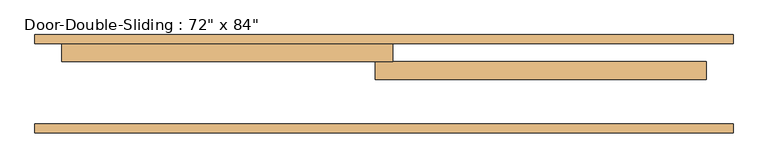
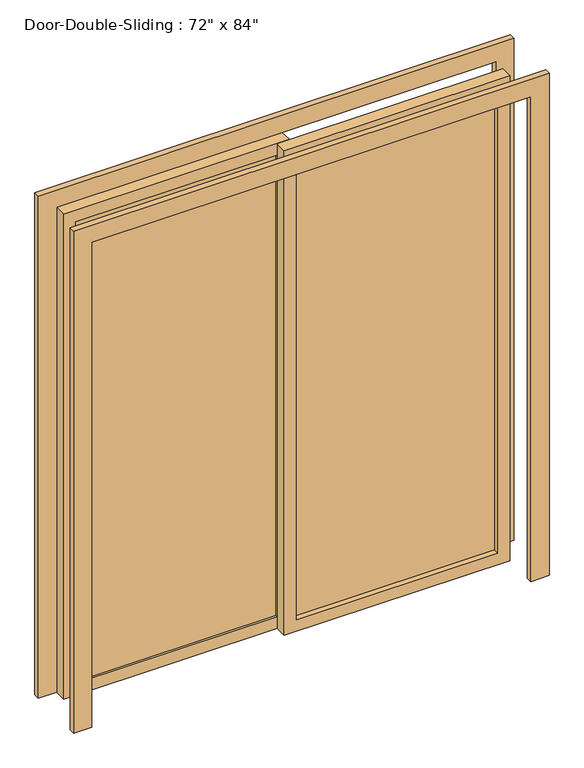
"""IFC4 building model written with IfcOpenShell, lengths in millimetres: door geometry."""

from ifc_helpers import new_model, si_unit, frame, origin, place, context, project, spatial, polyline, outline, extrude, source, transform, mapped, element, save


def door_d4d75d1e(model_context):
    return source(origin(), model_context, "Body", "SweptSolid", [
        extrude(outline(polyline([(0.0, 990.6), (2209.8, 990.6), (2209.8, -990.6), (0.0, -990.6), (0.0, -914.4), (2133.6, -914.4), (2133.6, 914.4), (0.0, 914.4), (0.0, 990.6)])), frame((0.0, 241.3, 0.0), z_axis=(0.0, 1.0, 0.0), x_axis=(0.0, 0.0, 1.0)), (0.0, 0.0, 1.0), 25.4),
        extrude(outline(polyline([(0.0, -990.6), (0.0, -914.4), (2133.6, -914.4), (2133.6, 914.4), (0.0, 914.4), (0.0, 990.6), (2209.8, 990.6), (2209.8, -990.6), (0.0, -990.6)])), frame((0.0, -12.7, 0.0), z_axis=(0.0, 1.0, 0.0), x_axis=(0.0, 0.0, 1.0)), (0.0, 0.0, 1.0), 25.4),
        extrude(outline(polyline([(2133.6, 25.4), (2133.6, -914.4), (0.0, -914.4), (0.0, 25.4), (2133.6, 25.4)]), holes=[polyline([(2082.8, -25.4), (50.8, -25.4), (50.8, -863.6), (2082.8, -863.6), (2082.8, -25.4)])]), frame((0.0, 190.5, 0.0), z_axis=(0.0, 1.0, 0.0), x_axis=(0.0, 0.0, 1.0)), (0.0, 0.0, 1.0), 50.8),
        extrude(outline(polyline([(2133.6, -25.4), (0.0, -25.4), (0.0, 914.4), (2133.6, 914.4), (2133.6, -25.4)]), holes=[polyline([(2082.8, 25.4), (2082.8, 863.6), (50.8, 863.6), (50.8, 25.4), (2082.8, 25.4)])]), frame((0.0, 139.7, 0.0), z_axis=(0.0, 1.0, 0.0), x_axis=(0.0, 0.0, 1.0)), (0.0, 0.0, 1.0), 50.8),
        extrude(outline(polyline([(-25.4, 200.025), (-863.6, 200.025), (-863.6, 206.375), (-25.4, 206.375), (-25.4, 200.025)])), frame((0.0, 0.0, 50.8), z_axis=(0.0, 0.0, 1.0), x_axis=(1.0, 0.0, 0.0)), (0.0, 0.0, 1.0), 2032.0),
        extrude(outline(polyline([(25.4, 168.275), (863.6, 168.275), (863.6, 161.925), (25.4, 161.925), (25.4, 168.275)])), frame((0.0, 0.0, 50.8), z_axis=(0.0, 0.0, 1.0), x_axis=(1.0, 0.0, 0.0)), (0.0, 0.0, 1.0), 2032.0),
    ])


if __name__ == "__main__":
    model = new_model("IFC4")
    model_context = context("Model", 3, world=origin())
    ifc_project = project(units=[si_unit("LENGTHUNIT", "METRE", prefix="MILLI")], contexts=[model_context])
    site = spatial("IfcSite", under=ifc_project)
    building = spatial("IfcBuilding", under=site)
    placement = place(None, origin())
    door_shape = door_d4d75d1e(model_context)
    element("IfcDoor", 1, ObjectType="Door-Double-Sliding : 72\" x 84\"", at=placement, inside=building, context=model_context, shape_type="MappedRepresentation", body=[
        mapped(door_shape, transform((0.0, 0.0, 0.0), x_axis=(1.0, 0.0, 0.0), y_axis=(0.0, 1.0, 0.0), z_axis=(0.0, 0.0, 1.0))),
    ])
    save(model, "model.ifc")

# Revit data of these elements
# Type "Door-Double-Sliding : 72\" x 84\""
#   Type Mark = "10"
#   Construction Type Id = "opn-d45"
#   Assembly Code = "C1020"
#   Analytic Construction = "Wood frame, double glass door "
#   Thickness = 0' - 2"
#   Thermal Resistance (R) = 1.8150 (h·ft²·°F)/BTU
#   Heat Transfer Coefficient (U) = 0.5510 BTU/(h·ft²·°F)
#   Height = 7' - 0"
#   Rail Width = 0' - 2"
#   Stiles = 0' - 2"
#   Trim Projection Ext = 0' - 1"
#   Trim Projection Int = 0' - 1"
#   Trim Width = 0' - 3"
#   Width = 6' - 0"
#   Define Thermal Properties by = 1
#   Glazing = Glass
#   Panel Material = Wood - Birch - Solid Stained Light Low Gloss
#   Trim Material = Paint - Sienna
#   Visual Light Transmittance = 0
#   Solar Heat Gain Coefficient = 0
#   Function = (empty or 0)
#   Wall Closure = (empty or 0)
# Element 1 (IfcDoor, "Door-Double-Sliding : 72\" x 84\"")
#   Materials on its faces: "Paint - Sienna", "Wood - Birch - Solid Stained Light Low Gloss", "Glass"
# Materials
#   "Glass": class "Glass", colour RGB 0 128 192, transparency 0.75, Description = "Soda Lime Glass", Cost = 0
#   "Wood - Birch - Solid Stained Light Low Gloss": class "Wood", colour RGB 210 159 95, transparency 0, Cost = 0
#   "Paint - Sienna": colour RGB 118 70 51, transparency 0, Cost = 0
